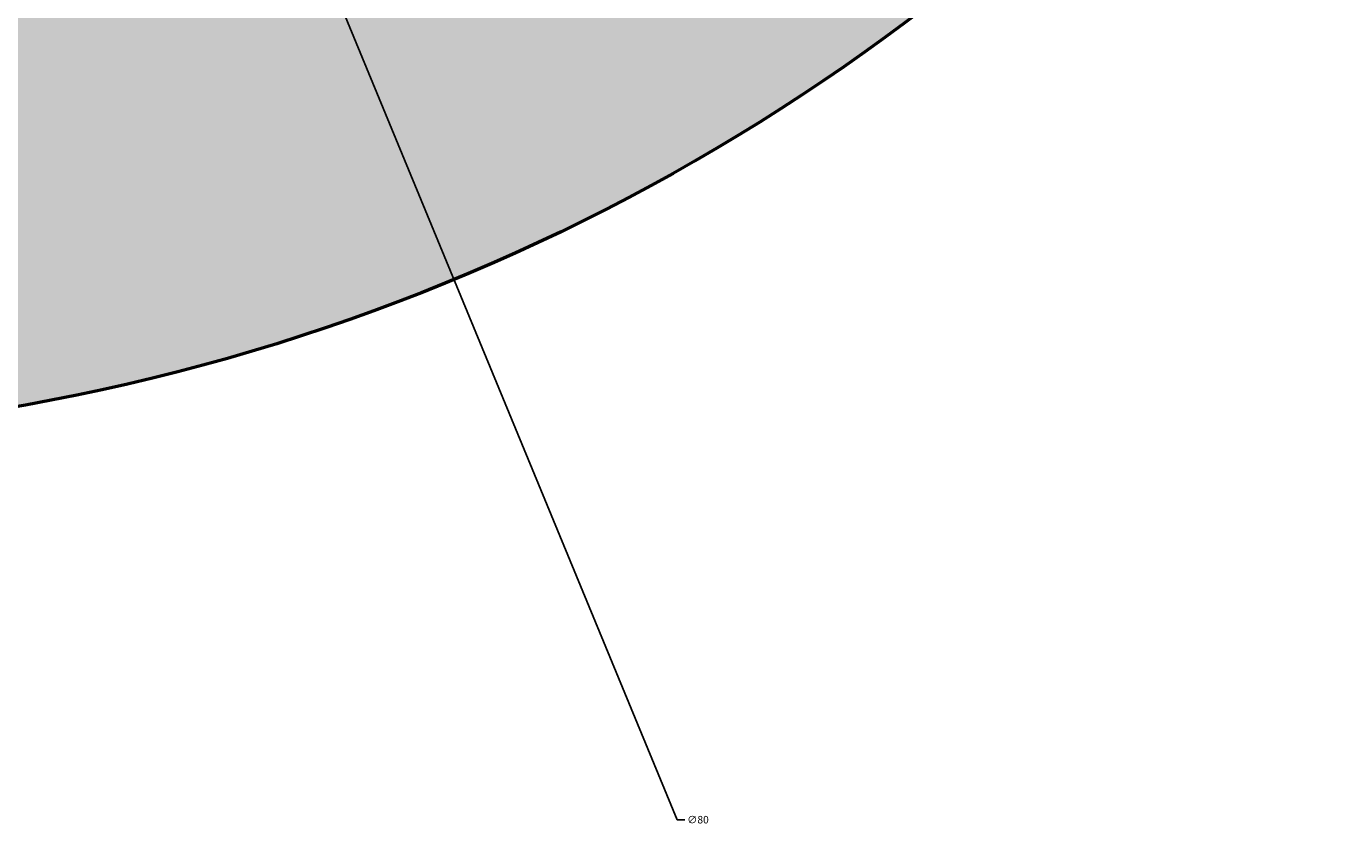
# Model space of a CAD drawing. Units: inches. Extents: x 139261 to 139415, y 52839 to 52963.
# Tile 10 of 20: x 139349 to 139381, y 52841 to 52860. Entities that reach past the tile are written whole.
import ezdxf

# ---------------------------------------------------------------- set-up
doc = ezdxf.new("R2010")
doc.units = ezdxf.units.IN
doc.header["$MEASUREMENT"] = 0
for name, color, linetype, lineweight in [('M-DIMS', 2, 'Continuous', 25), ('M-HATC', 8, 'Continuous', 18), ('M-OUTL', 7, 'Continuous', 50)]:
    doc.layers.add(name, color=color, linetype=linetype, lineweight=lineweight)
doc.styles.get("Standard").update_dxf_attribs({"font": 'arial.ttf'})
doc.dimstyles.get("Standard").update_dxf_attribs({"dimtxt": 0.18, "dimasz": 0.18, "dimexe": 0.18, "dimexo": 0.0625, "dimgap": 0.09, "dimtad": 0, "dimtih": 1, "dimtoh": 1, "dimdec": 4, "dimzin": 0, "dimdsep": 46, "dimtxsty": 'Standard', "dimcen": 0.09, "dimadec": 0, "dimazin": 0, "dimtfac": 1, "dimtdec": 4, "dimtofl": 0, "dimtmove": 0, "dimatfit": 3, "dimfxl": 1, "dimtolj": 1, "dimtzin": 0, "dimarcsym": 0})

# ---------------------------------------------------------------- blocks, each defined once
blk = doc.blocks.new('*D10')
at = {"layer": 'Defpoints', "color": 0, "transparency": 16777216}
for p in [(139325.07, 52937.181), (139355.644, 52863.254)]:
    blk.add_point(p, dxfattribs=at)
at = {"layer": 'M-DIMS', "color": 0, "lineweight": -2, "transparency": 16777216}
for p, q in [((139340.357, 52900.127), (139340.357, 52900.307)), ((139340.267, 52900.217), (139340.447, 52900.217)), ((139364.816, 52841.075), (139355.712, 52863.087)), ((139364.996, 52841.075), (139364.816, 52841.075))]:
    blk.add_line(p, q, dxfattribs=at)
at = {"layer": 'M-DIMS', "color": 0, "transparency": 16777216}
blk.add_solid([(139355.74, 52863.099), (139355.685, 52863.076), (139355.644, 52863.254)], dxfattribs=at)
at = {"layer": 'M-DIMS', "color": 0, "transparency": 16777216, "insert": (139365.312, 52841.075), "char_height": 0.18, "attachment_point": 5}
blk.add_mtext('\\A1;∅80', dxfattribs=at)

msp = doc.modelspace()

# ---------------------------------------------------------------- hatches: boundary and pattern name
at = {"layer": 'M-HATC'}
h = msp.add_hatch(color=256, dxfattribs=at)
h.dxf.hatch_style = 1
h.paths.add_polyline_path([(139290.35689, 52900.21749, 1), (139390.35689, 52900.21749, 1)])
h.paths.add_polyline_path([(139335.36666, 52939.90499, -0.01563646), (139335.35689, 52940.21749, -1), (139345.35689, 52940.21749, -0.01563646), (139345.34711, 52939.90499, -0.13461315), (139364.89157, 52931.80941, -0.691035), (139373.64116, 52928.50176, -0.21521822), (139371.94881, 52924.75216, -0.13461315), (139380.04439, 52905.20771, -0.43265224), (139385.35689, 52900.21749, -0.43265224), (139380.04439, 52895.22726, -0.13461315), (139371.94881, 52875.68281, -0.21521822), (139373.64116, 52871.93321, -0.691035), (139364.89157, 52868.62556, -0.13461315), (139345.34711, 52860.52999, -0.01563646), (139345.35689, 52860.21749, -1), (139335.35689, 52860.21749, -0.01563646), (139335.36666, 52860.52999, -0.13461315), (139315.82221, 52868.62556, -0.691035), (139307.07262, 52871.93321, -0.21521822), (139308.76496, 52875.68281, -0.13461315), (139300.66939, 52895.22726, -0.43265224), (139295.35689, 52900.21749, -0.43265224), (139300.66939, 52905.20771, -0.13461315), (139308.76496, 52924.75216, -0.21521822), (139307.07262, 52928.50176, -0.691035), (139315.82221, 52931.80941, -0.13461315)], flags=16)
h.paths.add_polyline_path([(139365.35689, 52900.21749, -1), (139315.35689, 52900.21749, -1)], flags=0)
h.paths.add_polyline_path([(139323.71474, 52911.30978), (139356.99903, 52911.30978, -0.3027197), (139356.99903, 52889.12519), (139323.71474, 52889.12519, -0.3027197)], flags=0)
h.paths.add_polyline_path([(139364.89157, 52931.80941, 0.13461315), (139345.34711, 52939.90499, -0.93933644), (139335.36666, 52939.90499, 0.13461315), (139315.82221, 52931.80941, -0.18270763), (139317.07262, 52928.50176, -0.64579494), (139308.76496, 52924.75216, 0.13461315), (139300.66939, 52905.20771, -0.39601219), (139305.35689, 52900.21749, -0.39601219), (139300.66939, 52895.22726, 0.13461315), (139308.76496, 52875.68281, -0.64579494), (139317.07262, 52871.93321, -0.18270763), (139315.82221, 52868.62556, 0.13461315), (139335.36666, 52860.52999, -0.93933644), (139345.34711, 52860.52999, 0.13461315), (139364.89157, 52868.62556, -0.18270763), (139363.64116, 52871.93321, -0.64579494), (139371.94881, 52875.68281, 0.13461315), (139380.04439, 52895.22726, -0.39601219), (139375.35689, 52900.21749, -0.39601219), (139380.04439, 52905.20771, 0.13461315), (139371.94881, 52924.75216, -0.64579494), (139363.64116, 52928.50176, -0.18270763)], flags=0)

# ---------------------------------------------------------------- linework, layer by layer
at = {"layer": 'M-OUTL'}
msp.add_circle((139340.35689, 52900.21749), 50, dxfattribs=at)

# ---------------------------------------------------------------- dimensions: what is measured, and where the dimension line sits
at = {"layer": 'M-DIMS'}
dim = msp.add_diameter_dim_2p(p1=(139325.07023, 52937.18123), p2=(139355.64354, 52863.25374), dimstyle='Standard', override={"dimdec": 0, "dimlfac": 1, "dimrnd": 0, "dimzin": 0, "dimdsep": 46, "dimlunit": 2}, dxfattribs=at)
dim.commit()
dim.dimension.update_dxf_attribs({"geometry": '*D10', "text_midpoint": (139365.31206, 52841.0755), "dimtype": 163})

doc.saveas('drawing.dxf')
